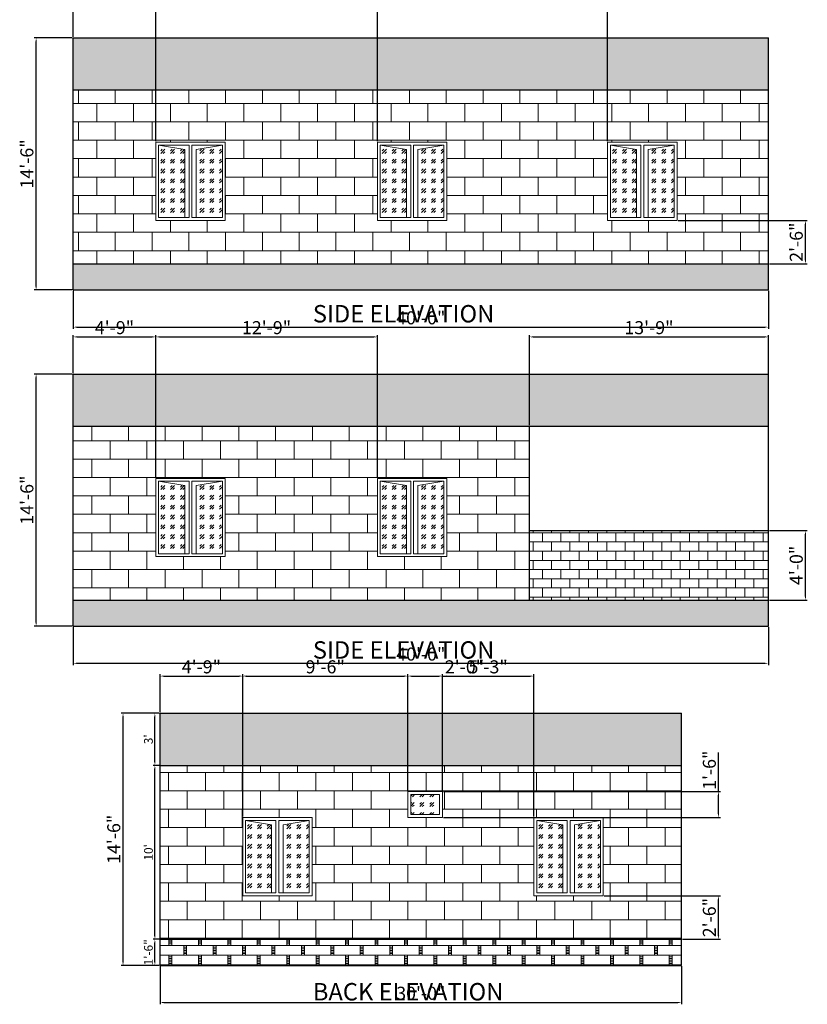
# Model space of a CAD drawing. Units: inches. Extents: x 2639 to 6021, y 292 to 2009.
# Tile 1 of 6: x 2639 to 3183, y 292 to 971. Entities that reach past the tile are written whole.
import ezdxf

# ---------------------------------------------------------------- set-up
doc = ezdxf.new("R2010")
doc.units = ezdxf.units.IN
for name, color, linetype, lineweight in [('A-ANNO-DIMS', 2, 'Continuous', 18), ('A-ANNO-TEXT', 7, 'Continuous', 18), ('A-ELEV', 7, 'Continuous', 30), ('A-ELEV-PATT', 8, 'Continuous', 13), ('A-GLAZ', 4, 'Continuous', 18), ('A-GLAZ-PATT', 9, 'Continuous', 13)]:
    doc.layers.add(name, color=color, linetype=linetype, lineweight=lineweight)
doc.layers.add('A-ELEV-MASN-PATT', color=30, linetype='Continuous', lineweight=13, true_color=0xf26722)
doc.styles.get("Standard").update_dxf_attribs({"font": 'arial.ttf'})
doc.dimstyles.new('ISO-25', dxfattribs={"dimtxt": 9, "dimasz": 2.5, "dimexe": 1.25, "dimexo": 0.625, "dimtad": 1, "dimdec": 1, "dimlunit": 3, "dimtxsty": 'Standard', "dimcen": 2.5, "dimadec": 0, "dimazin": 0, "dimtfac": 1, "dimtdec": 1, "dimtmove": 0, "dimatfit": 3, "dimfxl": 1, "dimarcsym": 0})

# ---------------------------------------------------------------- blocks, each defined once
blk = doc.blocks.new('*D18')
at = {"layer": 'A-ANNO-DIMS', "color": 0, "lineweight": -2, "transparency": 16777216}
for p, q in [((2735.48, 337.02), (2731.25, 337.02)), ((2732.5, 321.52), (2732.5, 334.52)), ((2735.48, 319.02), (2731.25, 319.02))]:
    blk.add_line(p, q, dxfattribs=at)
at = {"layer": 'A-ANNO-DIMS', "color": 0, "transparency": 16777216}
for points in [[(2732.09, 334.52), (2732.92, 334.52), (2732.5, 337.02)], [(2732.09, 321.52), (2732.92, 321.52), (2732.5, 319.02)]]:
    blk.add_solid(points, dxfattribs=at)
at = {"layer": 'Defpoints', "color": 0, "transparency": 16777216}
for p in [(2732.5, 337.02), (2736.11, 337.02), (2736.11, 319.02)]:
    blk.add_point(p, dxfattribs=at)
at = {"layer": 'A-ANNO-DIMS', "color": 0, "transparency": 16777216, "insert": (2728.81, 328.02), "char_height": 6, "attachment_point": 5, "rotation": 90}
blk.add_mtext('1\'-6"', dxfattribs=at)
blk = doc.blocks.new('*D19')
at = {"layer": 'A-ANNO-DIMS', "color": 0, "lineweight": -2, "transparency": 16777216}
for p, q in [((2735.48, 457.02), (2731.25, 457.02)), ((2732.5, 339.52), (2732.5, 454.52)), ((2735.48, 337.02), (2731.25, 337.02))]:
    blk.add_line(p, q, dxfattribs=at)
at = {"layer": 'A-ANNO-DIMS', "color": 0, "transparency": 16777216}
for points in [[(2732.09, 454.52), (2732.92, 454.52), (2732.5, 457.02)], [(2732.09, 339.52), (2732.92, 339.52), (2732.5, 337.02)]]:
    blk.add_solid(points, dxfattribs=at)
at = {"layer": 'Defpoints', "color": 0, "transparency": 16777216}
for p in [(2732.5, 457.02), (2736.11, 457.02), (2736.11, 337.02)]:
    blk.add_point(p, dxfattribs=at)
at = {"layer": 'A-ANNO-DIMS', "color": 0, "transparency": 16777216, "insert": (2728.81, 397.02), "char_height": 6, "attachment_point": 5, "rotation": 90}
blk.add_mtext("10'", dxfattribs=at)
blk = doc.blocks.new('*D20')
at = {"layer": 'A-ANNO-DIMS', "color": 0, "lineweight": -2, "transparency": 16777216}
for p, q in [((2735.48, 493.02), (2731.25, 493.02)), ((2732.5, 459.52), (2732.5, 490.52)), ((2735.48, 457.02), (2731.25, 457.02))]:
    blk.add_line(p, q, dxfattribs=at)
at = {"layer": 'A-ANNO-DIMS', "color": 0, "transparency": 16777216}
for points in [[(2732.09, 490.52), (2732.92, 490.52), (2732.5, 493.02)], [(2732.09, 459.52), (2732.92, 459.52), (2732.5, 457.02)]]:
    blk.add_solid(points, dxfattribs=at)
at = {"layer": 'Defpoints', "color": 0, "transparency": 16777216}
for p in [(2732.5, 493.02), (2736.11, 493.02), (2736.11, 457.02)]:
    blk.add_point(p, dxfattribs=at)
at = {"layer": 'A-ANNO-DIMS', "color": 0, "transparency": 16777216, "insert": (2728.81, 475.02), "char_height": 6, "attachment_point": 5, "rotation": 90}
blk.add_mtext("3'", dxfattribs=at)
blk = doc.blocks.new('*D78')
at = {"layer": 'A-ANNO-DIMS', "color": 0, "lineweight": -2, "transparency": 16777216}
for p, q in [((2736.11, 318.4), (2736.11, 292.17)), ((3096.11, 318.4), (3096.11, 292.17)), ((2738.61, 293.42), (3093.61, 293.42))]:
    blk.add_line(p, q, dxfattribs=at)
at = {"layer": 'A-ANNO-DIMS', "color": 0, "transparency": 16777216}
for points in [[(2738.61, 293.84), (2738.61, 293), (2736.11, 293.42)], [(3093.61, 293.84), (3093.61, 293), (3096.11, 293.42)]]:
    blk.add_solid(points, dxfattribs=at)
at = {"layer": 'Defpoints', "color": 0, "transparency": 16777216}
for p in [(2736.11, 319.02), (3096.11, 319.02), (3096.11, 293.42)]:
    blk.add_point(p, dxfattribs=at)
at = {"layer": 'A-ANNO-DIMS', "color": 0, "transparency": 16777216, "insert": (2916.11, 298.64), "char_height": 9, "attachment_point": 5}
blk.add_mtext('30\'-0"', dxfattribs=at)
blk = doc.blocks.new('*D79')
at = {"layer": 'A-ANNO-DIMS', "color": 0, "lineweight": -2, "transparency": 16777216}
for p, q in [((2735.48, 493.02), (2709.26, 493.02)), ((2710.51, 321.52), (2710.51, 490.52)), ((2735.48, 319.02), (2709.26, 319.02))]:
    blk.add_line(p, q, dxfattribs=at)
at = {"layer": 'A-ANNO-DIMS', "color": 0, "transparency": 16777216}
for points in [[(2710.09, 490.52), (2710.92, 490.52), (2710.51, 493.02)], [(2710.09, 321.52), (2710.92, 321.52), (2710.51, 319.02)]]:
    blk.add_solid(points, dxfattribs=at)
at = {"layer": 'Defpoints', "color": 0, "transparency": 16777216}
for p in [(2710.51, 493.02), (2736.11, 493.02), (2736.11, 319.02)]:
    blk.add_point(p, dxfattribs=at)
at = {"layer": 'A-ANNO-DIMS', "color": 0, "transparency": 16777216, "insert": (2705.29, 406.02), "char_height": 9, "attachment_point": 5, "rotation": 90}
blk.add_mtext('14\'-6"', dxfattribs=at)
blk = doc.blocks.new('*D80')
at = {"layer": 'A-ANNO-DIMS', "color": 0, "lineweight": -2, "transparency": 16777216}
for p, q in [((2736.11, 493.65), (2736.11, 519.87)), ((2738.61, 518.62), (2790.61, 518.62)), ((2793.11, 421.65), (2793.11, 519.87))]:
    blk.add_line(p, q, dxfattribs=at)
at = {"layer": 'A-ANNO-DIMS', "color": 0, "transparency": 16777216}
for points in [[(2738.61, 519.04), (2738.61, 518.2), (2736.11, 518.62)], [(2790.61, 519.04), (2790.61, 518.2), (2793.11, 518.62)]]:
    blk.add_solid(points, dxfattribs=at)
at = {"layer": 'Defpoints', "color": 0, "transparency": 16777216}
for p in [(2793.11, 518.62), (2736.11, 493.02), (2793.11, 421.02)]:
    blk.add_point(p, dxfattribs=at)
at = {"layer": 'A-ANNO-DIMS', "color": 0, "transparency": 16777216, "insert": (2764.61, 523.84), "char_height": 9, "attachment_point": 5}
blk.add_mtext('4\'-9"', dxfattribs=at)
blk = doc.blocks.new('*D81')
at = {"layer": 'A-ANNO-DIMS', "color": 0, "lineweight": -2, "transparency": 16777216}
for p, q in [((2793.11, 421.65), (2793.11, 519.87)), ((2795.61, 518.62), (2904.61, 518.62)), ((2907.11, 439.65), (2907.11, 519.87))]:
    blk.add_line(p, q, dxfattribs=at)
at = {"layer": 'A-ANNO-DIMS', "color": 0, "transparency": 16777216}
for points in [[(2795.61, 519.04), (2795.61, 518.2), (2793.11, 518.62)], [(2904.61, 519.04), (2904.61, 518.2), (2907.11, 518.62)]]:
    blk.add_solid(points, dxfattribs=at)
at = {"layer": 'Defpoints', "color": 0, "transparency": 16777216}
for p in [(2907.11, 518.62), (2907.11, 439.02), (2793.11, 421.02)]:
    blk.add_point(p, dxfattribs=at)
at = {"layer": 'A-ANNO-DIMS', "color": 0, "transparency": 16777216, "insert": (2850.11, 523.84), "char_height": 9, "attachment_point": 5}
blk.add_mtext('9\'-6"', dxfattribs=at)
blk = doc.blocks.new('*D82')
at = {"layer": 'A-ANNO-DIMS', "color": 0, "lineweight": -2, "transparency": 16777216}
for p, q in [((2907.11, 439.65), (2907.11, 519.87)), ((2909.61, 518.62), (2928.61, 518.62)), ((2931.11, 439.65), (2931.11, 519.87)), ((2931.11, 518.62), (2958.94, 518.62))]:
    blk.add_line(p, q, dxfattribs=at)
at = {"layer": 'A-ANNO-DIMS', "color": 0, "transparency": 16777216}
for points in [[(2909.61, 519.04), (2909.61, 518.2), (2907.11, 518.62)], [(2928.61, 519.04), (2928.61, 518.2), (2931.11, 518.62)]]:
    blk.add_solid(points, dxfattribs=at)
at = {"layer": 'Defpoints', "color": 0, "transparency": 16777216}
for p in [(2931.11, 518.62), (2907.11, 439.02), (2931.11, 439.02)]:
    blk.add_point(p, dxfattribs=at)
at = {"layer": 'A-ANNO-DIMS', "color": 0, "transparency": 16777216, "insert": (2946.27, 523.84), "char_height": 9, "attachment_point": 5}
blk.add_mtext('2\'-0"', dxfattribs=at)
blk = doc.blocks.new('*D83')
at = {"layer": 'A-ANNO-DIMS', "color": 0, "lineweight": -2, "transparency": 16777216}
for p, q in [((2931.11, 439.65), (2931.11, 519.87)), ((2933.61, 518.62), (2991.61, 518.62)), ((2994.11, 421.65), (2994.11, 519.87))]:
    blk.add_line(p, q, dxfattribs=at)
at = {"layer": 'A-ANNO-DIMS', "color": 0, "transparency": 16777216}
for points in [[(2933.61, 519.04), (2933.61, 518.2), (2931.11, 518.62)], [(2991.61, 519.04), (2991.61, 518.2), (2994.11, 518.62)]]:
    blk.add_solid(points, dxfattribs=at)
at = {"layer": 'Defpoints', "color": 0, "transparency": 16777216}
for p in [(2994.11, 518.62), (2931.11, 439.02), (2994.11, 421.02)]:
    blk.add_point(p, dxfattribs=at)
at = {"layer": 'A-ANNO-DIMS', "color": 0, "transparency": 16777216, "insert": (2962.61, 523.84), "char_height": 9, "attachment_point": 5}
blk.add_mtext('5\'-3"', dxfattribs=at)
blk = doc.blocks.new('*D84')
at = {"layer": 'A-ANNO-DIMS', "color": 0, "lineweight": -2, "transparency": 16777216}
for p, q in [((3121.71, 439.02), (3121.71, 465.85)), ((2931.73, 439.02), (3122.96, 439.02)), ((3121.71, 423.52), (3121.71, 436.52)), ((2931.73, 421.02), (3122.96, 421.02))]:
    blk.add_line(p, q, dxfattribs=at)
at = {"layer": 'A-ANNO-DIMS', "color": 0, "transparency": 16777216}
for points in [[(3121.29, 436.52), (3122.12, 436.52), (3121.71, 439.02)], [(3121.29, 423.52), (3122.12, 423.52), (3121.71, 421.02)]]:
    blk.add_solid(points, dxfattribs=at)
at = {"layer": 'Defpoints', "color": 0, "transparency": 16777216}
for p in [(2931.11, 439.02), (3121.71, 439.02), (2931.11, 421.02)]:
    blk.add_point(p, dxfattribs=at)
at = {"layer": 'A-ANNO-DIMS', "color": 0, "transparency": 16777216, "insert": (3116.49, 453.68), "char_height": 9, "attachment_point": 5, "rotation": 90}
blk.add_mtext('1\'-6"', dxfattribs=at)
blk = doc.blocks.new('*D85')
at = {"layer": 'A-ANNO-DIMS', "color": 0, "lineweight": -2, "transparency": 16777216}
for p, q in [((3042.73, 367.02), (3122.96, 367.02)), ((3121.71, 339.52), (3121.71, 364.52)), ((3096.73, 337.02), (3122.96, 337.02))]:
    blk.add_line(p, q, dxfattribs=at)
at = {"layer": 'A-ANNO-DIMS', "color": 0, "transparency": 16777216}
for points in [[(3121.29, 364.52), (3122.12, 364.52), (3121.71, 367.02)], [(3121.29, 339.52), (3122.12, 339.52), (3121.71, 337.02)]]:
    blk.add_solid(points, dxfattribs=at)
at = {"layer": 'Defpoints', "color": 0, "transparency": 16777216}
for p in [(3042.11, 367.02), (3121.71, 367.02), (3096.11, 337.02)]:
    blk.add_point(p, dxfattribs=at)
at = {"layer": 'A-ANNO-DIMS', "color": 0, "transparency": 16777216, "insert": (3116.49, 352.02), "char_height": 9, "attachment_point": 5, "rotation": 90}
blk.add_mtext('2\'-6"', dxfattribs=at)
blk = doc.blocks.new('*D86')
at = {"layer": 'A-ANNO-DIMS', "color": 0, "lineweight": -2, "transparency": 16777216}
for p, q in [((2676.11, 784.36), (2676.11, 758.14)), ((3156.11, 784.36), (3156.11, 758.14)), ((2678.61, 759.39), (3153.61, 759.39))]:
    blk.add_line(p, q, dxfattribs=at)
at = {"layer": 'A-ANNO-DIMS', "color": 0, "transparency": 16777216}
for points in [[(2678.61, 759.8), (2678.61, 758.97), (2676.11, 759.39)], [(3153.61, 759.8), (3153.61, 758.97), (3156.11, 759.39)]]:
    blk.add_solid(points, dxfattribs=at)
at = {"layer": 'Defpoints', "color": 0, "transparency": 16777216}
for p in [(2676.11, 784.99), (3156.11, 784.99), (3156.11, 759.39)]:
    blk.add_point(p, dxfattribs=at)
at = {"layer": 'A-ANNO-DIMS', "color": 0, "transparency": 16777216, "insert": (2916.11, 764.61), "char_height": 9, "attachment_point": 5}
blk.add_mtext('40\'-0"', dxfattribs=at)
blk = doc.blocks.new('*D87')
at = {"layer": 'A-ANNO-DIMS', "color": 0, "lineweight": -2, "transparency": 16777216}
for p, q in [((2675.48, 958.99), (2649.26, 958.99)), ((2650.51, 787.49), (2650.51, 956.49)), ((2675.48, 784.99), (2649.26, 784.99))]:
    blk.add_line(p, q, dxfattribs=at)
at = {"layer": 'A-ANNO-DIMS', "color": 0, "transparency": 16777216}
for points in [[(2650.09, 956.49), (2650.92, 956.49), (2650.51, 958.99)], [(2650.09, 787.49), (2650.92, 787.49), (2650.51, 784.99)]]:
    blk.add_solid(points, dxfattribs=at)
at = {"layer": 'Defpoints', "color": 0, "transparency": 16777216}
for p in [(2650.51, 958.99), (2676.11, 958.99), (2676.11, 784.99)]:
    blk.add_point(p, dxfattribs=at)
at = {"layer": 'A-ANNO-DIMS', "color": 0, "transparency": 16777216, "insert": (2645.29, 871.99), "char_height": 9, "attachment_point": 5, "rotation": 90}
blk.add_mtext('14\'-6"', dxfattribs=at)
blk = doc.blocks.new('*D88')
at = {"layer": 'A-ANNO-DIMS', "color": 0, "lineweight": -2, "transparency": 16777216}
for p, q in [((2676.11, 959.61), (2676.11, 985.84)), ((2733.11, 887.61), (2733.11, 985.84)), ((2678.61, 984.59), (2730.61, 984.59))]:
    blk.add_line(p, q, dxfattribs=at)
at = {"layer": 'A-ANNO-DIMS', "color": 0, "transparency": 16777216}
for points in [[(2678.61, 985), (2678.61, 984.17), (2676.11, 984.59)], [(2730.61, 985), (2730.61, 984.17), (2733.11, 984.59)]]:
    blk.add_solid(points, dxfattribs=at)
at = {"layer": 'Defpoints', "color": 0, "transparency": 16777216}
for p in [(2733.11, 984.59), (2676.11, 958.99), (2733.11, 886.99)]:
    blk.add_point(p, dxfattribs=at)
at = {"layer": 'A-ANNO-DIMS', "color": 0, "transparency": 16777216, "insert": (2704.61, 989.81), "char_height": 9, "attachment_point": 5}
blk.add_mtext('4\'-9"', dxfattribs=at)
blk = doc.blocks.new('*D89')
at = {"layer": 'A-ANNO-DIMS', "color": 0, "lineweight": -2, "transparency": 16777216}
for p, q in [((2733.11, 887.61), (2733.11, 985.84)), ((2886.11, 887.61), (2886.11, 985.84)), ((2735.61, 984.59), (2883.61, 984.59))]:
    blk.add_line(p, q, dxfattribs=at)
at = {"layer": 'A-ANNO-DIMS', "color": 0, "transparency": 16777216}
for points in [[(2735.61, 985), (2735.61, 984.17), (2733.11, 984.59)], [(2883.61, 985), (2883.61, 984.17), (2886.11, 984.59)]]:
    blk.add_solid(points, dxfattribs=at)
at = {"layer": 'Defpoints', "color": 0, "transparency": 16777216}
for p in [(2886.11, 984.59), (2733.11, 886.99), (2886.11, 886.99)]:
    blk.add_point(p, dxfattribs=at)
at = {"layer": 'A-ANNO-DIMS', "color": 0, "transparency": 16777216, "insert": (2809.61, 989.81), "char_height": 9, "attachment_point": 5}
blk.add_mtext('12\'-9"', dxfattribs=at)
blk = doc.blocks.new('*D90')
at = {"layer": 'A-ANNO-DIMS', "color": 0, "lineweight": -2, "transparency": 16777216}
for p, q in [((2886.11, 887.61), (2886.11, 985.84)), ((3045.11, 887.61), (3045.11, 985.84)), ((2888.61, 984.59), (3042.61, 984.59))]:
    blk.add_line(p, q, dxfattribs=at)
at = {"layer": 'A-ANNO-DIMS', "color": 0, "transparency": 16777216}
for points in [[(2888.61, 985), (2888.61, 984.17), (2886.11, 984.59)], [(3042.61, 985), (3042.61, 984.17), (3045.11, 984.59)]]:
    blk.add_solid(points, dxfattribs=at)
at = {"layer": 'Defpoints', "color": 0, "transparency": 16777216}
for p in [(3045.11, 984.59), (2886.11, 886.99), (3045.11, 886.99)]:
    blk.add_point(p, dxfattribs=at)
at = {"layer": 'A-ANNO-DIMS', "color": 0, "transparency": 16777216, "insert": (2965.61, 989.81), "char_height": 9, "attachment_point": 5}
blk.add_mtext('13\'-3"', dxfattribs=at)
blk = doc.blocks.new('*D91')
at = {"layer": 'A-ANNO-DIMS', "color": 0, "lineweight": -2, "transparency": 16777216}
for p, q in [((3093.73, 832.99), (3182.96, 832.99)), ((3181.71, 805.49), (3181.71, 830.49)), ((3156.73, 802.99), (3182.96, 802.99))]:
    blk.add_line(p, q, dxfattribs=at)
at = {"layer": 'A-ANNO-DIMS', "color": 0, "transparency": 16777216}
for points in [[(3181.29, 830.49), (3182.12, 830.49), (3181.71, 832.99)], [(3181.29, 805.49), (3182.12, 805.49), (3181.71, 802.99)]]:
    blk.add_solid(points, dxfattribs=at)
at = {"layer": 'Defpoints', "color": 0, "transparency": 16777216}
for p in [(3093.11, 832.99), (3181.71, 832.99), (3156.11, 802.99)]:
    blk.add_point(p, dxfattribs=at)
at = {"layer": 'A-ANNO-DIMS', "color": 0, "transparency": 16777216, "insert": (3176.49, 817.99), "char_height": 9, "attachment_point": 5, "rotation": 90}
blk.add_mtext('2\'-6"', dxfattribs=at)
blk = doc.blocks.new('*D92')
at = {"layer": 'A-ANNO-DIMS', "color": 0, "lineweight": -2, "transparency": 16777216}
for p, q in [((2676.11, 552.4), (2676.11, 526.17)), ((3156.11, 552.4), (3156.11, 526.17)), ((2678.61, 527.42), (3153.61, 527.42))]:
    blk.add_line(p, q, dxfattribs=at)
at = {"layer": 'A-ANNO-DIMS', "color": 0, "transparency": 16777216}
for points in [[(2678.61, 527.84), (2678.61, 527), (2676.11, 527.42)], [(3153.61, 527.84), (3153.61, 527), (3156.11, 527.42)]]:
    blk.add_solid(points, dxfattribs=at)
at = {"layer": 'Defpoints', "color": 0, "transparency": 16777216}
for p in [(2676.11, 553.02), (3156.11, 553.02), (3156.11, 527.42)]:
    blk.add_point(p, dxfattribs=at)
at = {"layer": 'A-ANNO-DIMS', "color": 0, "transparency": 16777216, "insert": (2916.11, 532.64), "char_height": 9, "attachment_point": 5}
blk.add_mtext('40\'-0"', dxfattribs=at)
blk = doc.blocks.new('*D93')
at = {"layer": 'A-ANNO-DIMS', "color": 0, "lineweight": -2, "transparency": 16777216}
for p, q in [((2675.48, 727.02), (2649.26, 727.02)), ((2650.51, 555.52), (2650.51, 724.52)), ((2675.48, 553.02), (2649.26, 553.02))]:
    blk.add_line(p, q, dxfattribs=at)
at = {"layer": 'A-ANNO-DIMS', "color": 0, "transparency": 16777216}
for points in [[(2650.09, 724.52), (2650.92, 724.52), (2650.51, 727.02)], [(2650.09, 555.52), (2650.92, 555.52), (2650.51, 553.02)]]:
    blk.add_solid(points, dxfattribs=at)
at = {"layer": 'Defpoints', "color": 0, "transparency": 16777216}
for p in [(2650.51, 727.02), (2676.11, 727.02), (2676.11, 553.02)]:
    blk.add_point(p, dxfattribs=at)
at = {"layer": 'A-ANNO-DIMS', "color": 0, "transparency": 16777216, "insert": (2645.29, 640.02), "char_height": 9, "attachment_point": 5, "rotation": 90}
blk.add_mtext('14\'-6"', dxfattribs=at)
blk = doc.blocks.new('*D94')
at = {"layer": 'A-ANNO-DIMS', "color": 0, "lineweight": -2, "transparency": 16777216}
for p, q in [((2676.11, 727.65), (2676.11, 753.87)), ((2678.61, 752.62), (2730.61, 752.62)), ((2733.11, 655.65), (2733.11, 753.87))]:
    blk.add_line(p, q, dxfattribs=at)
at = {"layer": 'A-ANNO-DIMS', "color": 0, "transparency": 16777216}
for points in [[(2678.61, 753.04), (2678.61, 752.2), (2676.11, 752.62)], [(2730.61, 753.04), (2730.61, 752.2), (2733.11, 752.62)]]:
    blk.add_solid(points, dxfattribs=at)
at = {"layer": 'Defpoints', "color": 0, "transparency": 16777216}
for p in [(2733.11, 752.62), (2676.11, 727.02), (2733.11, 655.02)]:
    blk.add_point(p, dxfattribs=at)
at = {"layer": 'A-ANNO-DIMS', "color": 0, "transparency": 16777216, "insert": (2704.61, 757.84), "char_height": 9, "attachment_point": 5}
blk.add_mtext('4\'-9"', dxfattribs=at)
blk = doc.blocks.new('*D95')
at = {"layer": 'A-ANNO-DIMS', "color": 0, "lineweight": -2, "transparency": 16777216}
for p, q in [((2733.11, 655.65), (2733.11, 753.87)), ((2735.61, 752.62), (2883.61, 752.62)), ((2886.11, 655.65), (2886.11, 753.87))]:
    blk.add_line(p, q, dxfattribs=at)
at = {"layer": 'A-ANNO-DIMS', "color": 0, "transparency": 16777216}
for points in [[(2735.61, 753.04), (2735.61, 752.2), (2733.11, 752.62)], [(2883.61, 753.04), (2883.61, 752.2), (2886.11, 752.62)]]:
    blk.add_solid(points, dxfattribs=at)
at = {"layer": 'Defpoints', "color": 0, "transparency": 16777216}
for p in [(2886.11, 752.62), (2733.11, 655.02), (2886.11, 655.02)]:
    blk.add_point(p, dxfattribs=at)
at = {"layer": 'A-ANNO-DIMS', "color": 0, "transparency": 16777216, "insert": (2809.61, 757.84), "char_height": 9, "attachment_point": 5}
blk.add_mtext('12\'-9"', dxfattribs=at)
blk = doc.blocks.new('*D96')
at = {"layer": 'A-ANNO-DIMS', "color": 0, "lineweight": -2, "transparency": 16777216}
for p, q in [((2991.11, 691.65), (2991.11, 753.87)), ((2993.61, 752.62), (3153.61, 752.62)), ((3156.11, 691.65), (3156.11, 753.87))]:
    blk.add_line(p, q, dxfattribs=at)
at = {"layer": 'A-ANNO-DIMS', "color": 0, "transparency": 16777216}
for points in [[(2993.61, 753.04), (2993.61, 752.2), (2991.11, 752.62)], [(3153.61, 753.04), (3153.61, 752.2), (3156.11, 752.62)]]:
    blk.add_solid(points, dxfattribs=at)
at = {"layer": 'Defpoints', "color": 0, "transparency": 16777216}
for p in [(3156.11, 752.62), (2991.11, 691.02), (3156.11, 691.02)]:
    blk.add_point(p, dxfattribs=at)
at = {"layer": 'A-ANNO-DIMS', "color": 0, "transparency": 16777216, "insert": (3073.61, 757.84), "char_height": 9, "attachment_point": 5}
blk.add_mtext('13\'-9"', dxfattribs=at)
blk = doc.blocks.new('*D97')
at = {"layer": 'A-ANNO-DIMS', "color": 0, "lineweight": -2, "transparency": 16777216}
for p, q in [((3156.73, 619.02), (3182.96, 619.02)), ((3181.71, 573.52), (3181.71, 616.52)), ((3156.73, 571.02), (3182.96, 571.02))]:
    blk.add_line(p, q, dxfattribs=at)
at = {"layer": 'A-ANNO-DIMS', "color": 0, "transparency": 16777216}
for points in [[(3181.29, 616.52), (3182.12, 616.52), (3181.71, 619.02)], [(3181.29, 573.52), (3182.12, 573.52), (3181.71, 571.02)]]:
    blk.add_solid(points, dxfattribs=at)
at = {"layer": 'Defpoints', "color": 0, "transparency": 16777216}
for p in [(3156.11, 619.02), (3181.71, 619.02), (3156.11, 571.02)]:
    blk.add_point(p, dxfattribs=at)
at = {"layer": 'A-ANNO-DIMS', "color": 0, "transparency": 16777216, "insert": (3176.49, 595.02), "char_height": 9, "attachment_point": 5, "rotation": 90}
blk.add_mtext('4\'-0"', dxfattribs=at)

msp = doc.modelspace()

# ---------------------------------------------------------------- hatches: boundary and pattern name
at = {"layer": 'A-ELEV-MASN-PATT'}
h = msp.add_hatch(dxfattribs=at)
h.set_pattern_fill('BRICK', color=256, scale=2)
h.set_pattern_definition([(0, (0, 12), (0, 12.7), []), (90, (0, 12), (-25.4, 2e-15), [12.7, -12.7]), (90, (12.7, 12), (-25.4, 2e-15), [-12.7, 12.7])])
h.paths.add_polyline_path([(2676.11, 802.99), (3156.11, 802.99), (3156.11, 922.99), (2676.11, 922.99)])
h.paths.add_polyline_path([(2733.11, 886.99), (2781.11, 886.99), (2781.11, 832.99), (2733.11, 832.99)], flags=16)
h.paths.add_polyline_path([(2735.11, 884.99), (2756.11, 884.99), (2756.11, 834.99), (2735.11, 834.99)], flags=0)
h.paths.add_polyline_path([(2758.11, 884.99), (2779.11, 884.99), (2779.11, 834.99), (2758.11, 834.99)], flags=0)
h.paths.add_polyline_path([(2886.11, 886.99), (2934.11, 886.99), (2934.11, 832.99), (2886.11, 832.99)], flags=16)
h.paths.add_polyline_path([(2888.11, 884.99), (2909.11, 884.99), (2909.11, 834.99), (2888.11, 834.99)], flags=0)
h.paths.add_polyline_path([(2911.11, 884.99), (2932.11, 884.99), (2932.11, 834.99), (2911.11, 834.99)], flags=0)
h.paths.add_polyline_path([(3045.11, 886.99), (3093.11, 886.99), (3093.11, 832.99), (3045.11, 832.99)], flags=16)
h.paths.add_polyline_path([(3047.11, 884.99), (3068.11, 884.99), (3068.11, 834.99), (3047.11, 834.99)], flags=0)
h.paths.add_polyline_path([(3070.11, 884.99), (3091.11, 884.99), (3091.11, 834.99), (3070.11, 834.99)], flags=0)
h = msp.add_hatch(dxfattribs=at)
h.set_pattern_fill('BRICK', color=256, scale=2)
h.set_pattern_definition([(0, (-2124.439, -804.88), (0, 12.7), []), (90, (-2124.44, -804.88), (-25.4, 2e-15), [12.7, -12.7]), (90, (-2111.74, -804.88), (-25.4, 2e-15), [-12.7, 12.7])])
h.paths.add_polyline_path([(2991.11, 691.02), (2676.11, 691.02), (2676.11, 571.02), (2991.11, 571.02)])
h.paths.add_polyline_path([(2934.11, 601.02), (2886.11, 601.02), (2886.11, 655.02), (2934.11, 655.02)], flags=16)
h.paths.add_polyline_path([(2932.11, 603.02), (2911.11, 603.02), (2911.11, 653.02), (2932.11, 653.02)], flags=0)
h.paths.add_polyline_path([(2909.11, 603.02), (2888.11, 603.02), (2888.11, 653.02), (2909.11, 653.02)], flags=0)
h.paths.add_polyline_path([(2781.11, 601.02), (2733.11, 601.02), (2733.11, 655.02), (2781.11, 655.02)], flags=16)
h.paths.add_polyline_path([(2779.11, 603.02), (2758.11, 603.02), (2758.11, 653.02), (2779.11, 653.02)], flags=0)
h.paths.add_polyline_path([(2756.11, 603.02), (2735.11, 603.02), (2735.11, 653.02), (2756.11, 653.02)], flags=0)
h = msp.add_hatch(dxfattribs=at)
h.set_pattern_fill('BRICK', color=256)
h.set_pattern_definition([(0, (-2124.439, -804.88), (0, 6.35), []), (90, (-2124.439, -804.88), (-12.7, 8e-16), [6.35, -6.35]), (90, (-2118.089, -804.88), (-12.7, 8e-16), [-6.35, 6.35])])
h.paths.add_polyline_path([(2991.11, 619.02), (2991.11, 571.02), (3156.11, 571.02), (3156.11, 619.02)])
h = msp.add_hatch(dxfattribs=at)
h.set_pattern_fill('BRICK', color=256, scale=2)
h.set_pattern_definition([(0, (-2820.598, -779.774), (0, 12.7), []), (90, (-2820.598, -779.774), (-25.4, 2e-15), [12.7, -12.7]), (90, (-2807.898, -779.774), (-25.4, 2e-15), [-12.7, 12.7])])
h.paths.add_polyline_path([(2736.11, 457.02), (2736.11, 337.02), (3096.11, 337.02), (3096.11, 457.02)])
h.paths.add_polyline_path([(2907.11, 439.02), (2931.11, 439.02), (2931.11, 421.02), (2907.11, 421.02)], flags=16)
h.paths.add_polyline_path([(2909.11, 437.02), (2929.11, 437.02), (2929.11, 423.02), (2909.11, 423.02)], flags=0)
h.paths.add_polyline_path([(2841.11, 421.02), (2841.11, 367.02), (2793.11, 367.02), (2793.11, 421.02)], flags=16)
h.paths.add_polyline_path([(2839.11, 419.02), (2839.11, 369.02), (2818.11, 369.02), (2818.11, 419.02)], flags=0)
h.paths.add_polyline_path([(2816.11, 419.02), (2816.11, 369.02), (2795.11, 369.02), (2795.11, 419.02)], flags=0)
h.paths.add_polyline_path([(2994.11, 421.02), (3042.11, 421.02), (3042.11, 367.02), (2994.11, 367.02)], flags=16)
h.paths.add_polyline_path([(2996.11, 419.02), (3017.11, 419.02), (3017.11, 369.02), (2996.11, 369.02)], flags=0)
h.paths.add_polyline_path([(3019.11, 419.02), (3040.11, 419.02), (3040.11, 369.02), (3019.11, 369.02)], flags=0)
at = {"layer": 'A-ELEV-PATT'}
h = msp.add_hatch(dxfattribs=at)
h.set_pattern_fill('STARS', color=256, scale=0.8)
h.set_pattern_definition([(0, (-2193.443, -234), (0, 4.399409), [2.54, -2.54]), (60, (-2193.443, -234), (-3.81, 2.1997045), [2.54, -2.54]), (120, (-2192.173, -231.8003), (-3.81, -2.1997045), [2.54, -2.54])])
h.paths.add_polyline_path([(2676.11, 958.99), (2676.11, 922.99), (3156.11, 922.99), (3156.11, 958.99)])
h = msp.add_hatch(dxfattribs=at)
h.set_pattern_fill('BRSTONE', color=256, scale=0.8)
h.set_pattern_definition([(0, (-2193.443, -234), (0, 6.7056), []), (90, (-2175.155, -234), (-10.16, 6.7056), [6.7056, -6.7056]), (90, (-2177.187, -234), (-10.16, 6.7056), [6.7056, -6.7056]), (0, (-2175.155, -232.8824), (10.16, 6.7056), [-18.288, 2.032]), (0, (-2175.155, -231.765), (10.16, 6.7056), [-18.288, 2.032]), (0, (-2175.155, -230.647), (10.16, 6.7056), [-18.288, 2.032]), (0, (-2175.155, -229.5296), (10.16, 6.7056), [-18.288, 2.032]), (0, (-2175.155, -228.412), (10.16, 6.7056), [-18.288, 2.032])])
h.paths.add_polyline_path([(3156.11, 784.99), (3156.11, 802.99), (2676.11, 802.99), (2676.11, 784.99)])
h = msp.add_hatch(dxfattribs=at)
h.set_pattern_fill('STARS', color=256, scale=0.8)
h.set_pattern_definition([(0, (-2193.443, -465.9667), (0, 4.399409), [2.54, -2.54]), (60, (-2193.443, -465.9667), (-3.81, 2.1997045), [2.54, -2.54]), (120, (-2192.173, -463.767), (-3.81, -2.1997045), [2.54, -2.54])])
h.paths.add_polyline_path([(2676.11, 727.02), (2676.11, 691.02), (3156.11, 691.02), (3156.11, 727.02)])
h = msp.add_hatch(dxfattribs=at)
h.set_pattern_fill('BRSTONE', color=256, scale=0.8)
h.set_pattern_definition([(0, (-2193.443, -465.967), (0, 6.7056), []), (90, (-2175.155, -465.967), (-10.16, 6.7056), [6.7056, -6.7056]), (90, (-2177.187, -465.967), (-10.16, 6.7056), [6.7056, -6.7056]), (0, (-2175.155, -464.849), (10.16, 6.7056), [-18.288, 2.032]), (0, (-2175.155, -463.7315), (10.16, 6.7056), [-18.288, 2.032]), (0, (-2175.155, -462.614), (10.16, 6.7056), [-18.288, 2.032]), (0, (-2175.155, -461.496), (10.16, 6.7056), [-18.288, 2.032]), (0, (-2175.155, -460.379), (10.16, 6.7056), [-18.288, 2.032])])
h.paths.add_polyline_path([(3156.11, 553.02), (3156.11, 571.02), (2676.11, 571.02), (2676.11, 553.02)])
h = msp.add_hatch(dxfattribs=at)
h.set_pattern_fill('STARS', color=256, scale=0.8)
h.set_pattern_definition([(0, (-1561.548, -699.9667), (0, 4.399409), [2.54, -2.54]), (60, (-1561.548, -699.9667), (-3.81, 2.1997045), [2.54, -2.54]), (120, (-1560.278, -697.767), (-3.81, -2.1997045), [2.54, -2.54])])
h.paths.add_polyline_path([(2736.11, 493.02), (2736.11, 457.02), (3096.11, 457.02), (3096.11, 493.02)])
h = msp.add_hatch(dxfattribs=at)
h.set_pattern_fill('BRSTONE', color=256, scale=0.8)
h.set_pattern_definition([(0, (-1561.548, -699.967), (0, 6.7056), []), (90, (-1543.26, -699.967), (-10.16, 6.7056), [6.7056, -6.7056]), (90, (-1545.292, -699.967), (-10.16, 6.7056), [6.7056, -6.7056]), (0, (-1543.26, -698.849), (10.16, 6.7056), [-18.288, 2.032]), (0, (-1543.26, -697.7315), (10.16, 6.7056), [-18.288, 2.032]), (0, (-1543.26, -696.614), (10.16, 6.7056), [-18.288, 2.032]), (0, (-1543.26, -695.496), (10.16, 6.7056), [-18.288, 2.032]), (0, (-1543.26, -694.379), (10.16, 6.7056), [-18.288, 2.032])])
h.paths.add_polyline_path([(2736.11, 337.02), (2736.11, 319.02), (3096.11, 319.02), (3096.11, 337.02)])
at = {"layer": 'A-GLAZ-PATT'}
h = msp.add_hatch(dxfattribs=at)
h.set_pattern_fill('GOST_GLASS', color=256, scale=0.8)
h.set_pattern_definition([(45, (-1621.548, -234), (6.788225, 0), [4, -5.6]), (45, (-1619.851, -234), (6.788225, 0), [1.6, -8]), (45, (-1621.548, -232.303), (6.788225, 0), [1.6, -8])])
h.paths.add_polyline_path([(2753.11, 881.99), (2735.11, 884.99), (2735.11, 834.99), (2753.11, 834.99)])
h.paths.add_polyline_path([(2761.11, 834.99), (2779.11, 834.99), (2779.11, 884.99), (2761.11, 881.99)])
h = msp.add_hatch(dxfattribs=at)
h.set_pattern_fill('GOST_GLASS', color=256, scale=0.8)
h.set_pattern_definition([(45, (-1468.548, -234), (6.788225, 0), [4, -5.6]), (45, (-1466.851, -234), (6.788225, 0), [1.6, -8]), (45, (-1468.548, -232.303), (6.788225, 0), [1.6, -8])])
h.paths.add_polyline_path([(2906.11, 881.99), (2888.11, 884.99), (2888.11, 834.99), (2906.11, 834.99)])
h.paths.add_polyline_path([(2914.11, 834.99), (2932.11, 834.99), (2932.11, 884.99), (2914.11, 881.99)])
h = msp.add_hatch(dxfattribs=at)
h.set_pattern_fill('GOST_GLASS', color=256, scale=0.8)
h.set_pattern_definition([(45, (-1309.548, -234), (6.788225, 0), [4, -5.6]), (45, (-1307.851, -234), (6.788225, 0), [1.6, -8]), (45, (-1309.548, -232.303), (6.788225, 0), [1.6, -8])])
h.paths.add_polyline_path([(3065.11, 881.99), (3047.11, 884.99), (3047.11, 834.99), (3065.11, 834.99)])
h.paths.add_polyline_path([(3073.11, 834.99), (3091.11, 834.99), (3091.11, 884.99), (3073.11, 881.99)])
h = msp.add_hatch(dxfattribs=at)
h.set_pattern_fill('GOST_GLASS', color=256, scale=0.8)
h.set_pattern_definition([(45, (-1621.548, -465.9667), (6.788225, 0), [4, -5.6]), (45, (-1619.851, -465.9667), (6.788225, 0), [1.6, -8]), (45, (-1621.548, -464.2696), (6.788225, 0), [1.6, -8])])
h.paths.add_polyline_path([(2753.11, 650.02), (2735.11, 653.02), (2735.11, 603.02), (2753.11, 603.02)])
h.paths.add_polyline_path([(2761.11, 603.02), (2779.11, 603.02), (2779.11, 653.02), (2761.11, 650.02)])
h = msp.add_hatch(dxfattribs=at)
h.set_pattern_fill('GOST_GLASS', color=256, scale=0.8)
h.set_pattern_definition([(45, (-1468.548, -465.9667), (6.788225, 0), [4, -5.6]), (45, (-1466.851, -465.9667), (6.788225, 0), [1.6, -8]), (45, (-1468.548, -464.2696), (6.788225, 0), [1.6, -8])])
h.paths.add_polyline_path([(2906.11, 650.02), (2888.11, 653.02), (2888.11, 603.02), (2906.11, 603.02)])
h.paths.add_polyline_path([(2914.11, 603.02), (2932.11, 603.02), (2932.11, 653.02), (2914.11, 650.02)])
h = msp.add_hatch(dxfattribs=at)
h.set_pattern_fill('GOST_GLASS', color=256, scale=0.8)
h.set_pattern_definition([(45, (-2820.598, -779.7735), (6.788225, 0), [4, -5.6]), (45, (-2818.901, -779.7735), (6.788225, 0), [1.6, -8]), (45, (-2820.598, -778.0764), (6.788225, 0), [1.6, -8])])
h.paths.add_polyline_path([(2909.11, 423.02), (2929.11, 423.02), (2929.11, 437.02), (2909.11, 437.02)])
h = msp.add_hatch(dxfattribs=at)
h.set_pattern_fill('GOST_GLASS', color=256, scale=0.8)
h.set_pattern_definition([(45, (-1561.548, -699.9667), (6.788225, 0), [4, -5.6]), (45, (-1559.851, -699.9667), (6.788225, 0), [1.6, -8]), (45, (-1561.548, -698.2696), (6.788225, 0), [1.6, -8])])
h.paths.add_polyline_path([(2813.11, 416.02), (2795.11, 419.02), (2795.11, 369.02), (2813.11, 369.02)])
h.paths.add_polyline_path([(2821.11, 369.02), (2839.11, 369.02), (2839.11, 419.02), (2821.11, 416.02)])
h = msp.add_hatch(dxfattribs=at)
h.set_pattern_fill('GOST_GLASS', color=256, scale=0.8)
h.set_pattern_definition([(45, (-1360.548, -699.9667), (6.788225, 0), [4, -5.6]), (45, (-1358.851, -699.9667), (6.788225, 0), [1.6, -8]), (45, (-1360.548, -698.2696), (6.788225, 0), [1.6, -8])])
h.paths.add_polyline_path([(3014.11, 416.02), (2996.11, 419.02), (2996.11, 369.02), (3014.11, 369.02)])
h.paths.add_polyline_path([(3022.11, 369.02), (3040.11, 369.02), (3040.11, 419.02), (3022.11, 416.02)])

# ---------------------------------------------------------------- linework, layer by layer
at = {"layer": 'A-ELEV'}
for p, q in [((2676.11, 784.99), (2676.11, 958.99)), ((2676.11, 958.99), (3156.11, 958.99)), ((3156.11, 784.99), (3156.11, 958.99)), ((2676.11, 922.99), (3156.11, 922.99)), ((2676.11, 802.99), (3156.11, 802.99)), ((2676.11, 784.99), (3156.11, 784.99)), ((2676.11, 553.02), (2676.11, 727.02)), ((2676.11, 727.02), (3156.11, 727.02)), ((3156.11, 553.02), (3156.11, 727.02)), ((2676.11, 691.02), (3156.11, 691.02)), ((2991.11, 571.02), (2991.11, 691.02)), ((2991.11, 619.02), (3156.11, 619.02)), ((2676.11, 571.02), (3156.11, 571.02)), ((2676.11, 553.02), (3156.11, 553.02)), ((2736.11, 319.02), (2736.11, 493.02)), ((2736.11, 493.02), (3096.11, 493.02)), ((3096.11, 319.02), (3096.11, 493.02)), ((2736.11, 457.02), (3096.11, 457.02)), ((2736.11, 337.02), (3096.11, 337.02)), ((2736.11, 319.02), (3096.11, 319.02))]:
    msp.add_line(p, q, dxfattribs=at)
at = {"layer": 'A-GLAZ'}
for p, q in [((2733.11, 832.99), (2733.11, 886.99)), ((2733.11, 886.99), (2781.11, 886.99)), ((2735.11, 834.99), (2735.11, 884.99)), ((2735.11, 884.99), (2756.11, 884.99)), ((2735.11, 884.99), (2753.11, 881.99)), ((2756.11, 884.99), (2756.11, 834.99)), ((2758.11, 884.99), (2779.11, 884.99)), ((2758.11, 884.99), (2758.11, 834.99)), ((2761.11, 881.99), (2779.11, 884.99)), ((2779.11, 834.99), (2779.11, 884.99)), ((2781.11, 832.99), (2781.11, 886.99)), ((2886.11, 832.99), (2886.11, 886.99)), ((2886.11, 886.99), (2934.11, 886.99)), ((2888.11, 834.99), (2888.11, 884.99)), ((2888.11, 884.99), (2909.11, 884.99)), ((2888.11, 884.99), (2906.11, 881.99)), ((2909.11, 884.99), (2909.11, 834.99)), ((2911.11, 884.99), (2932.11, 884.99)), ((2911.11, 884.99), (2911.11, 834.99)), ((2914.11, 881.99), (2932.11, 884.99)), ((2932.11, 834.99), (2932.11, 884.99)), ((2934.11, 832.99), (2934.11, 886.99)), ((3045.11, 832.99), (3045.11, 886.99)), ((3045.11, 886.99), (3093.11, 886.99)), ((3047.11, 834.99), (3047.11, 884.99)), ((3047.11, 884.99), (3068.11, 884.99)), ((3047.11, 884.99), (3065.11, 881.99)), ((3068.11, 884.99), (3068.11, 834.99)), ((3070.11, 884.99), (3091.11, 884.99)), ((3070.11, 884.99), (3070.11, 834.99)), ((3073.11, 881.99), (3091.11, 884.99)), ((3091.11, 834.99), (3091.11, 884.99)), ((3093.11, 832.99), (3093.11, 886.99)), ((2753.11, 881.99), (2753.11, 834.99)), ((2761.11, 881.99), (2761.11, 834.99)), ((2906.11, 881.99), (2906.11, 834.99)), ((2914.11, 881.99), (2914.11, 834.99)), ((3065.11, 881.99), (3065.11, 834.99)), ((3073.11, 881.99), (3073.11, 834.99)), ((2733.11, 832.99), (2781.11, 832.99)), ((2735.11, 834.99), (2756.11, 834.99)), ((2758.11, 834.99), (2779.11, 834.99)), ((2886.11, 832.99), (2934.11, 832.99)), ((2888.11, 834.99), (2909.11, 834.99)), ((2911.11, 834.99), (2932.11, 834.99)), ((3045.11, 832.99), (3093.11, 832.99)), ((3047.11, 834.99), (3068.11, 834.99)), ((3070.11, 834.99), (3091.11, 834.99)), ((2733.11, 601.02), (2733.11, 655.02)), ((2733.11, 655.02), (2781.11, 655.02)), ((2735.11, 603.02), (2735.11, 653.02)), ((2735.11, 653.02), (2756.11, 653.02)), ((2735.11, 653.02), (2753.11, 650.02)), ((2756.11, 653.02), (2756.11, 603.02)), ((2758.11, 653.02), (2779.11, 653.02)), ((2758.11, 653.02), (2758.11, 603.02)), ((2761.11, 650.02), (2779.11, 653.02)), ((2779.11, 603.02), (2779.11, 653.02)), ((2781.11, 601.02), (2781.11, 655.02)), ((2886.11, 601.02), (2886.11, 655.02)), ((2886.11, 655.02), (2934.11, 655.02)), ((2888.11, 603.02), (2888.11, 653.02)), ((2888.11, 653.02), (2909.11, 653.02)), ((2888.11, 653.02), (2906.11, 650.02)), ((2909.11, 653.02), (2909.11, 603.02)), ((2911.11, 653.02), (2932.11, 653.02)), ((2911.11, 653.02), (2911.11, 603.02)), ((2914.11, 650.02), (2932.11, 653.02)), ((2932.11, 603.02), (2932.11, 653.02)), ((2934.11, 601.02), (2934.11, 655.02)), ((2753.11, 650.02), (2753.11, 603.02)), ((2761.11, 650.02), (2761.11, 603.02)), ((2906.11, 650.02), (2906.11, 603.02)), ((2914.11, 650.02), (2914.11, 603.02)), ((2733.11, 601.02), (2781.11, 601.02)), ((2735.11, 603.02), (2756.11, 603.02)), ((2758.11, 603.02), (2779.11, 603.02)), ((2886.11, 601.02), (2934.11, 601.02)), ((2888.11, 603.02), (2909.11, 603.02)), ((2911.11, 603.02), (2932.11, 603.02)), ((2907.11, 439.02), (2907.11, 421.02)), ((2907.11, 439.02), (2931.11, 439.02)), ((2909.11, 437.02), (2909.11, 423.02)), ((2909.11, 437.02), (2929.11, 437.02)), ((2929.11, 437.02), (2929.11, 423.02)), ((2931.11, 439.02), (2931.11, 421.02)), ((2909.11, 423.02), (2929.11, 423.02)), ((2793.11, 367.02), (2793.11, 421.02)), ((2793.11, 421.02), (2841.11, 421.02)), ((2795.11, 369.02), (2795.11, 419.02)), ((2795.11, 419.02), (2816.11, 419.02)), ((2795.11, 419.02), (2813.11, 416.02)), ((2813.11, 416.02), (2813.11, 369.02)), ((2816.11, 419.02), (2816.11, 369.02)), ((2818.11, 419.02), (2839.11, 419.02)), ((2818.11, 419.02), (2818.11, 369.02)), ((2821.11, 416.02), (2839.11, 419.02)), ((2821.11, 416.02), (2821.11, 369.02)), ((2839.11, 369.02), (2839.11, 419.02)), ((2841.11, 367.02), (2841.11, 421.02)), ((2907.11, 421.02), (2931.11, 421.02)), ((2994.11, 367.02), (2994.11, 421.02)), ((2994.11, 421.02), (3042.11, 421.02)), ((2996.11, 369.02), (2996.11, 419.02)), ((2996.11, 419.02), (3017.11, 419.02)), ((2996.11, 419.02), (3014.11, 416.02)), ((3014.11, 416.02), (3014.11, 369.02)), ((3017.11, 419.02), (3017.11, 369.02)), ((3019.11, 419.02), (3040.11, 419.02)), ((3019.11, 419.02), (3019.11, 369.02)), ((3022.11, 416.02), (3040.11, 419.02)), ((3022.11, 416.02), (3022.11, 369.02)), ((3040.11, 369.02), (3040.11, 419.02)), ((3042.11, 367.02), (3042.11, 421.02)), ((2793.11, 367.02), (2841.11, 367.02)), ((2795.11, 369.02), (2816.11, 369.02)), ((2818.11, 369.02), (2839.11, 369.02)), ((2994.11, 367.02), (3042.11, 367.02)), ((2996.11, 369.02), (3017.11, 369.02)), ((3019.11, 369.02), (3040.11, 369.02))]:
    msp.add_line(p, q, dxfattribs=at)

# ---------------------------------------------------------------- texts
at = {"layer": 'A-ANNO-TEXT', "char_height": 12, "attachment_point": 1}
for s, insert in [('{\\fTimes New Roman|b0|i0|c0|p18;SIDE ELEVATION}', (2841.56, 774.61)), ('{\\fTimes New Roman|b0|i0|c0|p18;SIDE ELEVATION}', (2841.56, 542.65)), ('{\\fTimes New Roman|b0|i0|c0|p18;BACK ELEVATION}', (2841.56, 306.85))]:
    msp.add_mtext_dynamic_manual_height_columns(s, width=172.2916, gutter_width=12.5, heights=[0], dxfattribs=dict(at, insert=insert))

# ---------------------------------------------------------------- dimensions: what is measured, and where the dimension line sits
at = {"layer": 'A-ANNO-DIMS'}
for base, p1, p2, picture, middle in [((2733.11, 984.59), (2676.11, 958.99), (2733.11, 886.99), '*D88', (2704.61, 989.81)), ((2886.11, 984.59), (2733.11, 886.99), (2886.11, 886.99), '*D89', (2809.61, 989.81)), ((3045.11, 984.59), (2886.11, 886.99), (3045.11, 886.99), '*D90', (2965.61, 989.81)), ((3156.11, 759.39), (2676.11, 784.99), (3156.11, 784.99), '*D86', (2916.11, 764.61)), ((2733.11, 752.62), (2676.11, 727.02), (2733.11, 655.02), '*D94', (2704.61, 757.84)), ((2886.11, 752.62), (2733.11, 655.02), (2886.11, 655.02), '*D95', (2809.61, 757.84)), ((3156.11, 752.62), (2991.11, 691.02), (3156.11, 691.02), '*D96', (3073.61, 757.84)), ((3156.11, 527.42), (2676.11, 553.02), (3156.11, 553.02), '*D92', (2916.11, 532.64)), ((2793.11, 518.62), (2736.11, 493.02), (2793.11, 421.02), '*D80', (2764.61, 523.84)), ((2907.11, 518.62), (2793.11, 421.02), (2907.11, 439.02), '*D81', (2850.11, 523.84)), ((2931.11, 518.62), (2907.11, 439.02), (2931.11, 439.02), '*D82', (2946.27, 523.84)), ((2994.11, 518.62), (2931.11, 439.02), (2994.11, 421.02), '*D83', (2962.61, 523.84)), ((3096.11, 293.42), (2736.11, 319.02), (3096.11, 319.02), '*D78', (2916.11, 298.64))]:
    dim = msp.add_linear_dim(base=base, p1=p1, p2=p2, dimstyle='ISO-25', override={"dimdec": 1, "dimlfac": 1, "dimrnd": 0, "dimzin": 1, "dimdsep": 46, "dimlunit": 4, "dimfrac": 2}, dxfattribs=at)
    dim.commit()
    dim.dimension.update_dxf_attribs({"geometry": picture, "text_midpoint": middle})
for base, p1, p2, override, picture, middle in [((2650.51, 958.99), (2676.11, 784.99), (2676.11, 958.99), {"dimdec": 1, "dimlfac": 1, "dimrnd": 0, "dimzin": 1, "dimdsep": 46, "dimlunit": 4, "dimfrac": 2}, '*D87', (2645.29, 871.99)), ((3181.71, 832.99), (3156.11, 802.99), (3093.11, 832.99), {"dimdec": 1, "dimlfac": 1, "dimrnd": 0, "dimzin": 1, "dimdsep": 46, "dimlunit": 4, "dimfrac": 2}, '*D91', (3176.49, 817.99)), ((2650.51, 727.02), (2676.11, 553.02), (2676.11, 727.02), {"dimdec": 1, "dimlfac": 1, "dimrnd": 0, "dimzin": 1, "dimdsep": 46, "dimlunit": 4, "dimfrac": 2}, '*D93', (2645.29, 640.02)), ((3181.71, 619.02), (3156.11, 571.02), (3156.11, 619.02), {"dimdec": 1, "dimlfac": 1, "dimrnd": 0, "dimzin": 1, "dimdsep": 46, "dimlunit": 4, "dimfrac": 2}, '*D97', (3176.49, 595.02)), ((2710.51, 493.02), (2736.11, 319.02), (2736.11, 493.02), {"dimdec": 1, "dimlfac": 1, "dimrnd": 0, "dimzin": 1, "dimdsep": 46, "dimlunit": 4, "dimfrac": 2}, '*D79', (2705.29, 406.02)), ((2732.5, 493.02), (2736.11, 457.02), (2736.11, 493.02), {"dimtxt": 6, "dimclrd": 0, "dimclre": 0, "dimclrt": 0, "dimtmove": 1}, '*D20', (2728.81, 475.02)), ((3121.71, 439.02), (2931.11, 421.02), (2931.11, 439.02), {"dimdec": 1, "dimlfac": 1, "dimrnd": 0, "dimzin": 1, "dimdsep": 46, "dimlunit": 4, "dimfrac": 2}, '*D84', (3116.49, 453.68)), ((2732.5, 457.02), (2736.11, 337.02), (2736.11, 457.02), {"dimtxt": 6, "dimclrd": 0, "dimclre": 0, "dimclrt": 0, "dimtmove": 1}, '*D19', (2728.81, 397.02)), ((3121.71, 367.02), (3096.11, 337.02), (3042.11, 367.02), {"dimdec": 1, "dimlfac": 1, "dimrnd": 0, "dimzin": 1, "dimdsep": 46, "dimlunit": 4, "dimfrac": 2}, '*D85', (3116.49, 352.02)), ((2732.5, 337.02), (2736.11, 319.02), (2736.11, 337.02), {"dimtxt": 6, "dimclrd": 0, "dimclre": 0, "dimclrt": 0}, '*D18', (2728.81, 328.02))]:
    dim = msp.add_linear_dim(base=base, p1=p1, p2=p2, angle=90, dimstyle='ISO-25', override=override, dxfattribs=at)
    dim.commit()
    dim.dimension.update_dxf_attribs({"geometry": picture, "text_midpoint": middle})

doc.saveas('drawing.dxf')
